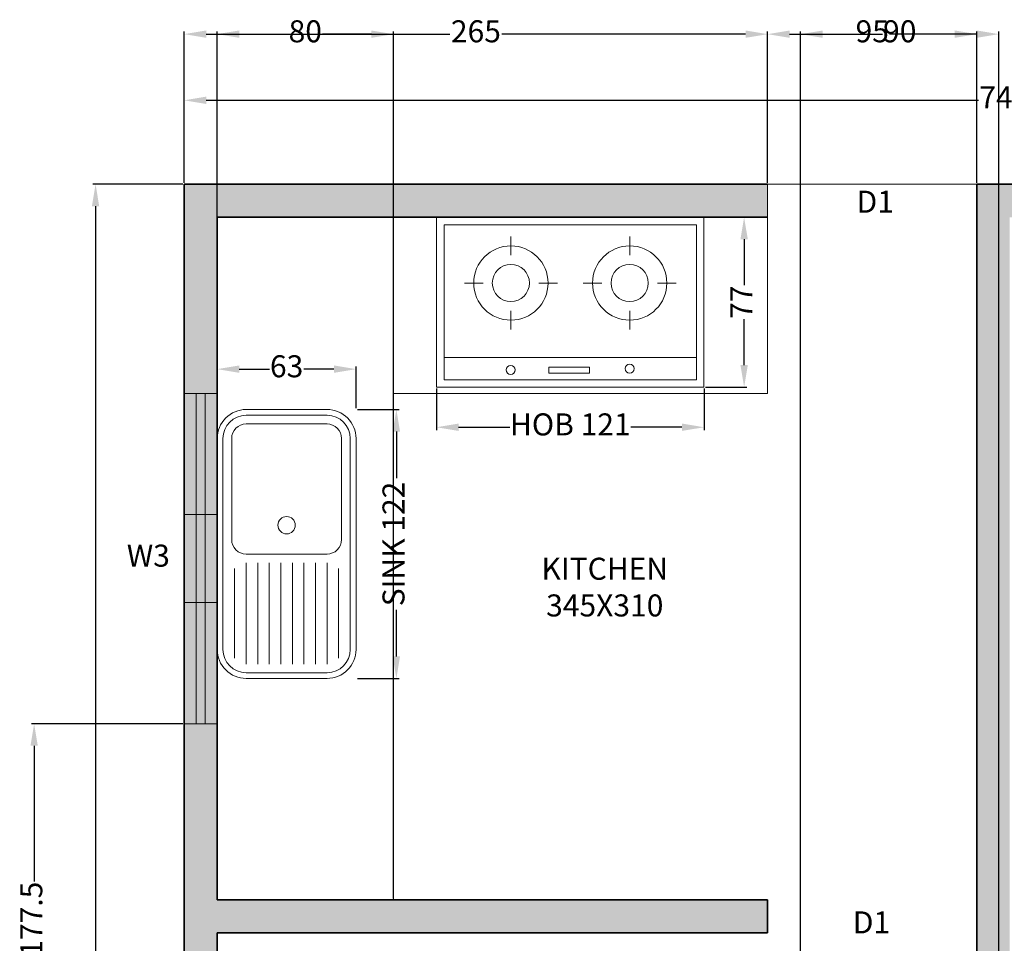
# Model space of a CAD drawing. Units: centimetres. Extents: x 2401 to 3632, y 2122 to 3526.
# Tile 8 of 10: x 2426 to 2873, y 3106 to 3526. Entities that reach past the tile are written whole.
import ezdxf

# ---------------------------------------------------------------- set-up
doc = ezdxf.new("R2010")
doc.units = ezdxf.units.CM
for name, color, linetype, lineweight in [('A-ANNO-DIMS', 9, 'Continuous', 18), ('A-ANNO-TEXT', 9, 'Continuous', 18), ('A-AREA-IDEN', 9, 'Continuous', 25), ('A-DOOR', 4, 'Continuous', 18), ('A-FLOR-CASE', 7, 'Continuous', 18), ('A-FLOR-FIXT', 9, 'Continuous', 18), ('A-GLAZ', 4, 'Continuous', 18), ('A-WALL', 7, 'Continuous', 35), ('equipments', 9, 'Continuous', 18)]:
    doc.layers.add(name, color=color, linetype=linetype, lineweight=lineweight)
doc.layers.add('A-GLAZ-PATT', color=251, linetype='Continuous', lineweight=13, true_color=0x636466)
doc.layers.add('A-WALL-PATT', color=18, linetype='Continuous', lineweight=13, true_color=0x000000)
doc.styles.get("Standard").update_dxf_attribs({"font": 'arial.ttf'})
doc.dimstyles.new('ISO-25', dxfattribs={"dimtxt": 10, "dimasz": 10, "dimexe": 1.25, "dimexo": 0.625, "dimtad": 0, "dimtxsty": 'Standard', "dimcen": 2.5, "dimadec": 0, "dimazin": 0, "dimtfac": 1, "dimtmove": 0, "dimatfit": 3, "dimfxl": 1, "dimarcsym": 0})

# ---------------------------------------------------------------- blocks, each defined once
blk = doc.blocks.new('cooktop_2')
at = {"color": 0}
for p, q in [((2566.17, 3601.98), (2636.16, 3601.98)), ((2566.17, 3601.98), (2566.17, 3557.53)), ((2568.12, 3600.04), (2634.22, 3600.04)), ((2568.12, 3600.04), (2568.12, 3559.48)), ((2634.22, 3600.04), (2634.22, 3559.48)), ((2636.16, 3601.98), (2636.16, 3557.53)), ((2585.62, 3596.92), (2585.62, 3592.06)), ((2616.72, 3596.92), (2616.72, 3592.06)), ((2573.47, 3584.77), (2578.33, 3584.77)), ((2592.91, 3584.77), (2597.78, 3584.77)), ((2604.56, 3584.77), (2609.42, 3584.77)), ((2624.01, 3584.77), (2628.87, 3584.77)), ((2585.62, 3577.47), (2585.62, 3572.61)), ((2616.72, 3577.47), (2616.72, 3572.61)), ((2568.12, 3565.31), (2634.22, 3565.31)), ((2595.51, 3561.18), (2595.51, 3562.73)), ((2595.51, 3562.73), (2606.23, 3562.73)), ((2606.23, 3562.73), (2606.23, 3561.18)), ((2568.12, 3559.48), (2634.22, 3559.48)), ((2606.23, 3561.18), (2595.51, 3561.18)), ((2566.17, 3557.53), (2636.16, 3557.53))]:
    blk.add_line(p, q, dxfattribs=at)
for centre, radius in [((2585.62, 3584.77), 9.72), ((2616.72, 3584.77), 9.72), ((2585.62, 3584.77), 4.86), ((2616.72, 3584.77), 4.86), ((2585.57, 3562.04), 1.17), ((2616.7, 3562.38), 1.17)]:
    blk.add_circle(centre, radius, dxfattribs=at)
blk = doc.blocks.new('v')
blk.add_blockref('cooktop_2', (0, 0))
blk = doc.blocks.new('SINK_KITCHEN_SNGL')
for p, q in [((-36.5, -2), (36.5, -2)), ((-39.5, -6), (-8.5, -6)), ((-44.5, -38), (-44.5, -10)), ((-41.5, -10), (-6.5, -10)), ((44.5, -10), (44.5, -38)), ((-41.5, -14), (-6.5, -14)), ((-41.5, -18), (-6.5, -18)), ((-41.5, -22), (-6.5, -22)), ((-41.5, -26), (-6.5, -26)), ((-41.5, -30), (-6.5, -30)), ((-41.5, -34), (-6.5, -34)), ((-41.5, -38), (-6.5, -38)), ((-39.5, -42), (-8.5, -42)), ((36.5, -46), (-36.5, -46))]:
    blk.add_line(p, q)
at = {"flags": 128}
for points in [[(36.5, 0, -0.414214), (46.5, -10), (46.5, -38, -0.414214), (36.5, -48), (-36.5, -48, -0.414214), (-46.5, -38), (-46.5, -10, -0.414214), (-36.5, 0)], [(36.5, -5, -0.414214), (41.5, -10), (41.5, -38, -0.414214), (36.5, -43), (1.5, -43, -0.414214), (-3.5, -38), (-3.5, -10, -0.414214), (1.5, -5)]]:
    blk.add_lwpolyline(points, format="xyb", close=True, dxfattribs=at)
blk.add_circle((6.5, -24), 3)
for centre, start, end in [((-36.5, -10), 90, 180), ((36.5, -10), 0, 90), ((-36.5, -38), 180, 270), ((36.5, -38), 270, 0)]:
    blk.add_arc(centre, 8, start, end)
blk = doc.blocks.new('*D12')
at = {"layer": 'A-ANNO-DIMS', "color": 0, "lineweight": -2, "transparency": 16777216}
for p, q in [((2499.81, 3451.1), (2458.94, 3451.1)), ((2460.19, 3441.1), (2460.19, 2873.73)), ((2460.19, 2276.1), (2460.19, 2843.48)), ((2499.81, 2266.1), (2458.94, 2266.1))]:
    blk.add_line(p, q, dxfattribs=at)
at = {"layer": 'A-ANNO-DIMS', "color": 0, "transparency": 16777216}
for points in [[(2458.52, 3441.1), (2461.85, 3441.1), (2460.19, 3451.1)], [(2458.52, 2276.1), (2461.85, 2276.1), (2460.19, 2266.1)]]:
    blk.add_solid(points, dxfattribs=at)
at = {"layer": 'Defpoints', "color": 0, "transparency": 16777216}
for p in [(2500.44, 3451.1), (2460.19, 2266.1), (2500.44, 2266.1)]:
    blk.add_point(p, dxfattribs=at)
at = {"layer": 'A-ANNO-DIMS', "color": 0, "transparency": 16777216, "insert": (2460.19, 2858.6), "char_height": 10, "attachment_point": 5, "rotation": 90}
blk.add_mtext('1185', dxfattribs=at)
blk = doc.blocks.new('*D17')
at = {"layer": 'A-ANNO-DIMS', "color": 0, "lineweight": -2, "transparency": 16777216}
for p, q in [((2500.44, 3451.73), (2500.44, 3490.46)), ((2510.44, 3489.21), (2861.27, 3489.21)), ((3235.44, 3489.21), (2884.6, 3489.21)), ((3245.44, 3451.73), (3245.44, 3490.46))]:
    blk.add_line(p, q, dxfattribs=at)
at = {"layer": 'A-ANNO-DIMS', "color": 0, "transparency": 16777216}
for points in [[(2510.44, 3490.88), (2510.44, 3487.55), (2500.44, 3489.21)], [(3235.44, 3490.88), (3235.44, 3487.55), (3245.44, 3489.21)]]:
    blk.add_solid(points, dxfattribs=at)
at = {"layer": 'Defpoints', "color": 0, "transparency": 16777216}
for p in [(3245.44, 3489.21), (2500.44, 3451.1), (3245.44, 3451.1)]:
    blk.add_point(p, dxfattribs=at)
at = {"layer": 'A-ANNO-DIMS', "color": 0, "transparency": 16777216, "insert": (2872.94, 3489.21), "char_height": 10, "attachment_point": 5}
blk.add_mtext('745', dxfattribs=at)
blk = doc.blocks.new('WIN-1500-3P')
for p, q in [((0, 15), (0, 0)), ((55, 15), (55, 0)), ((95, 15), (95, 0)), ((150, 15), (150, 0)), ((0, 9.5), (150, 9.5)), ((0, 5.5), (150, 5.5))]:
    blk.add_line(p, q)
blk = doc.blocks.new('*D28')
at = {"layer": 'A-ANNO-DIMS', "color": 0, "lineweight": -2, "transparency": 16777216}
for p, q in [((2615.07, 3358.34), (2615.07, 3339.49)), ((2736.54, 3358.34), (2736.54, 3339.49)), ((2625.07, 3340.74), (2648.29, 3340.74)), ((2726.54, 3340.74), (2703.32, 3340.74))]:
    blk.add_line(p, q, dxfattribs=at)
at = {"layer": 'A-ANNO-DIMS', "color": 0, "transparency": 16777216}
for points in [[(2625.07, 3342.41), (2625.07, 3339.08), (2615.07, 3340.74)], [(2726.54, 3342.41), (2726.54, 3339.08), (2736.54, 3340.74)]]:
    blk.add_solid(points, dxfattribs=at)
at = {"layer": 'Defpoints', "color": 0, "transparency": 16777216}
for p in [(2615.07, 3358.97), (2736.54, 3358.97), (2736.54, 3340.74)]:
    blk.add_point(p, dxfattribs=at)
at = {"layer": 'A-ANNO-DIMS', "color": 0, "transparency": 16777216, "insert": (2675.81, 3340.74), "char_height": 10, "attachment_point": 5}
blk.add_mtext('HOB 121', dxfattribs=at)
blk = doc.blocks.new('*D29')
at = {"layer": 'A-ANNO-DIMS', "color": 0, "lineweight": -2, "transparency": 16777216}
for p, q in [((2737.16, 3436.1), (2756.01, 3436.1)), ((2754.76, 3426.1), (2754.76, 3405.28)), ((2754.76, 3368.97), (2754.76, 3389.79)), ((2737.16, 3358.97), (2756.01, 3358.97))]:
    blk.add_line(p, q, dxfattribs=at)
at = {"layer": 'A-ANNO-DIMS', "color": 0, "transparency": 16777216}
for points in [[(2753.09, 3426.1), (2756.43, 3426.1), (2754.76, 3436.1)], [(2753.09, 3368.97), (2756.43, 3368.97), (2754.76, 3358.97)]]:
    blk.add_solid(points, dxfattribs=at)
at = {"layer": 'Defpoints', "color": 0, "transparency": 16777216}
for p in [(2736.54, 3436.1), (2754.76, 3436.1), (2736.54, 3358.97)]:
    blk.add_point(p, dxfattribs=at)
at = {"layer": 'A-ANNO-DIMS', "color": 0, "transparency": 16777216, "insert": (2754.76, 3397.53), "char_height": 10, "attachment_point": 5, "rotation": 90}
blk.add_mtext('77', dxfattribs=at)
blk = doc.blocks.new('*D30')
at = {"layer": 'A-ANNO-DIMS', "color": 0, "lineweight": -2, "transparency": 16777216}
for p, q in [((2579.1, 3348.81), (2598.05, 3348.81)), ((2596.8, 3338.81), (2596.8, 3317.58)), ((2596.8, 3236.66), (2596.8, 3257.89)), ((2579.1, 3226.66), (2598.05, 3226.66))]:
    blk.add_line(p, q, dxfattribs=at)
at = {"layer": 'A-ANNO-DIMS', "color": 0, "transparency": 16777216}
for points in [[(2595.14, 3338.81), (2598.47, 3338.81), (2596.8, 3348.81)], [(2595.14, 3236.66), (2598.47, 3236.66), (2596.8, 3226.66)]]:
    blk.add_solid(points, dxfattribs=at)
at = {"layer": 'Defpoints', "color": 0, "transparency": 16777216}
for p in [(2578.48, 3348.81), (2596.8, 3348.81), (2578.48, 3226.66)]:
    blk.add_point(p, dxfattribs=at)
at = {"layer": 'A-ANNO-DIMS', "color": 0, "transparency": 16777216, "insert": (2596.8, 3287.73), "char_height": 10, "attachment_point": 5, "rotation": 90}
blk.add_mtext('SINK 122', dxfattribs=at)
blk = doc.blocks.new('*D31')
at = {"layer": 'A-ANNO-DIMS', "color": 0, "lineweight": -2, "transparency": 16777216}
for p, q in [((2515.44, 3349.43), (2515.44, 3368.38)), ((2578.48, 3349.43), (2578.48, 3368.38)), ((2525.44, 3367.13), (2539.14, 3367.13)), ((2568.48, 3367.13), (2554.77, 3367.13))]:
    blk.add_line(p, q, dxfattribs=at)
at = {"layer": 'A-ANNO-DIMS', "color": 0, "transparency": 16777216}
for points in [[(2525.44, 3368.8), (2525.44, 3365.46), (2515.44, 3367.13)], [(2568.48, 3368.8), (2568.48, 3365.46), (2578.48, 3367.13)]]:
    blk.add_solid(points, dxfattribs=at)
at = {"layer": 'Defpoints', "color": 0, "transparency": 16777216}
for p in [(2515.44, 3367.13), (2515.44, 3348.81), (2578.48, 3348.81)]:
    blk.add_point(p, dxfattribs=at)
at = {"layer": 'A-ANNO-DIMS', "color": 0, "transparency": 16777216, "insert": (2546.96, 3367.13), "char_height": 10, "attachment_point": 5}
blk.add_mtext('63', dxfattribs=at)
blk = doc.blocks.new('*D42')
at = {"layer": 'A-ANNO-DIMS', "color": 0, "lineweight": -2, "transparency": 16777216}
for p, q in [((2499.81, 3206.1), (2431.04, 3206.1)), ((2432.29, 3196.1), (2432.29, 3134.42)), ((2432.29, 3038.6), (2432.29, 3100.29)), ((2499.81, 3028.6), (2431.04, 3028.6))]:
    blk.add_line(p, q, dxfattribs=at)
at = {"layer": 'A-ANNO-DIMS', "color": 0, "transparency": 16777216}
for points in [[(2430.62, 3196.1), (2433.95, 3196.1), (2432.29, 3206.1)], [(2430.62, 3038.6), (2433.95, 3038.6), (2432.29, 3028.6)]]:
    blk.add_solid(points, dxfattribs=at)
at = {"layer": 'Defpoints', "color": 0, "transparency": 16777216}
for p in [(2432.29, 3206.1), (2500.44, 3206.1), (2500.44, 3028.6)]:
    blk.add_point(p, dxfattribs=at)
at = {"layer": 'A-ANNO-DIMS', "color": 0, "transparency": 16777216, "insert": (2432.29, 3117.35), "char_height": 10, "attachment_point": 5, "rotation": 90}
blk.add_mtext('177.5', dxfattribs=at)
blk = doc.blocks.new('*D48')
at = {"layer": 'A-ANNO-DIMS', "color": 0, "lineweight": -2, "transparency": 16777216}
for p, q in [((2765.44, 3451.73), (2765.44, 3520.5)), ((2860.44, 3451.73), (2860.44, 3520.5)), ((2775.44, 3519.25), (2805.11, 3519.25)), ((2850.44, 3519.25), (2820.76, 3519.25))]:
    blk.add_line(p, q, dxfattribs=at)
at = {"layer": 'A-ANNO-DIMS', "color": 0, "transparency": 16777216}
for points in [[(2775.44, 3520.92), (2775.44, 3517.59), (2765.44, 3519.25)], [(2850.44, 3520.92), (2850.44, 3517.59), (2860.44, 3519.25)]]:
    blk.add_solid(points, dxfattribs=at)
at = {"layer": 'Defpoints', "color": 0, "transparency": 16777216}
for p in [(2860.44, 3519.25), (2765.44, 3451.1), (2860.44, 3451.1)]:
    blk.add_point(p, dxfattribs=at)
at = {"layer": 'A-ANNO-DIMS', "color": 0, "transparency": 16777216, "insert": (2812.94, 3519.25), "char_height": 10, "attachment_point": 5}
blk.add_mtext('95', dxfattribs=at)
blk = doc.blocks.new('*D49')
at = {"layer": 'A-ANNO-DIMS', "color": 0, "lineweight": -2, "transparency": 16777216}
for p, q in [((2500.44, 3451.73), (2500.44, 3520.5)), ((2765.44, 3451.73), (2765.44, 3520.5)), ((2510.44, 3519.25), (2621.14, 3519.25)), ((2755.44, 3519.25), (2644.73, 3519.25))]:
    blk.add_line(p, q, dxfattribs=at)
at = {"layer": 'A-ANNO-DIMS', "color": 0, "transparency": 16777216}
for points in [[(2510.44, 3520.92), (2510.44, 3517.59), (2500.44, 3519.25)], [(2755.44, 3520.92), (2755.44, 3517.59), (2765.44, 3519.25)]]:
    blk.add_solid(points, dxfattribs=at)
at = {"layer": 'Defpoints', "color": 0, "transparency": 16777216}
for p in [(2765.44, 3519.25), (2500.44, 3451.1), (2765.44, 3451.1)]:
    blk.add_point(p, dxfattribs=at)
at = {"layer": 'A-ANNO-DIMS', "color": 0, "transparency": 16777216, "insert": (2632.94, 3519.25), "char_height": 10, "attachment_point": 5}
blk.add_mtext('265', dxfattribs=at)
blk = doc.blocks.new('*D51')
at = {"layer": 'A-ANNO-DIMS', "color": 0, "lineweight": -2, "transparency": 16777216}
for p, q in [((2780.44, 2796.73), (2780.44, 3520.5)), ((2870.44, 2796.73), (2870.44, 3520.5)), ((2790.44, 3519.25), (2817.67, 3519.25)), ((2860.44, 3519.25), (2833.21, 3519.25))]:
    blk.add_line(p, q, dxfattribs=at)
at = {"layer": 'A-ANNO-DIMS', "color": 0, "transparency": 16777216}
for points in [[(2790.44, 3520.92), (2790.44, 3517.59), (2780.44, 3519.25)], [(2860.44, 3520.92), (2860.44, 3517.59), (2870.44, 3519.25)]]:
    blk.add_solid(points, dxfattribs=at)
at = {"layer": 'Defpoints', "color": 0, "transparency": 16777216}
for p in [(2870.44, 3519.25), (2780.44, 2796.1), (2870.44, 2796.1)]:
    blk.add_point(p, dxfattribs=at)
at = {"layer": 'A-ANNO-DIMS', "color": 0, "transparency": 16777216, "insert": (2825.44, 3519.25), "char_height": 10, "attachment_point": 5}
blk.add_mtext('90', dxfattribs=at)
blk = doc.blocks.new('*D53')
at = {"layer": 'A-ANNO-DIMS', "color": 0, "lineweight": -2, "transparency": 16777216}
for p, q in [((2515.44, 3126.73), (2515.44, 3520.5)), ((2595.44, 3126.73), (2595.44, 3520.5)), ((2525.44, 3519.25), (2547.66, 3519.25)), ((2585.44, 3519.25), (2563.21, 3519.25))]:
    blk.add_line(p, q, dxfattribs=at)
at = {"layer": 'A-ANNO-DIMS', "color": 0, "transparency": 16777216}
for points in [[(2525.44, 3520.92), (2525.44, 3517.59), (2515.44, 3519.25)], [(2585.44, 3520.92), (2585.44, 3517.59), (2595.44, 3519.25)]]:
    blk.add_solid(points, dxfattribs=at)
at = {"layer": 'Defpoints', "color": 0, "transparency": 16777216}
for p in [(2595.44, 3519.25), (2515.44, 3126.1), (2595.44, 3126.1)]:
    blk.add_point(p, dxfattribs=at)
at = {"layer": 'A-ANNO-DIMS', "color": 0, "transparency": 16777216, "insert": (2555.44, 3519.25), "char_height": 10, "attachment_point": 5}
blk.add_mtext('80', dxfattribs=at)

msp = doc.modelspace()

# ---------------------------------------------------------------- hatches: boundary and pattern name
at = {"layer": 'A-GLAZ-PATT'}
h = msp.add_hatch(color=256, dxfattribs=at)
h.dxf.hatch_style = 1
h.paths.add_polyline_path([(2505.936, 3356.104), (2500.436, 3356.104), (2500.436, 3301.104), (2505.936, 3301.104)])
h.paths.add_polyline_path([(2509.936, 3356.104), (2505.936, 3356.104), (2505.936, 3301.104), (2509.936, 3301.104)])
h.paths.add_polyline_path([(2515.436, 3335.674), (2515.436, 3356.104), (2509.936, 3356.104), (2509.936, 3301.104), (2515.436, 3301.104)])
h.paths.add_polyline_path([(2509.936, 3301.104), (2505.936, 3301.104), (2505.936, 3261.104), (2509.936, 3261.104)])
h.paths.add_polyline_path([(2515.436, 3301.104), (2509.936, 3301.104), (2509.936, 3261.104), (2515.436, 3261.104)])
h.paths.add_polyline_path([(2505.936, 3301.104), (2500.436, 3301.104), (2500.436, 3261.104), (2505.936, 3261.104)])
h.paths.add_polyline_path([(2515.436, 3261.104), (2509.936, 3261.104), (2509.936, 3206.104), (2515.436, 3206.104)])
h.paths.add_polyline_path([(2505.936, 3261.104), (2500.436, 3261.104), (2500.436, 3206.104), (2505.936, 3206.104)])
h.paths.add_polyline_path([(2509.936, 3261.104), (2505.936, 3261.104), (2505.936, 3206.104), (2509.936, 3206.104)])
h.paths.add_polyline_path([(3127.936, 3451.104), (3072.936, 3451.104), (3072.936, 3445.604), (3127.936, 3445.604)])
h.paths.add_polyline_path([(3032.936, 3441.604), (2977.936, 3441.604), (2977.936, 3436.104), (3032.936, 3436.104)])
h.paths.add_polyline_path([(3032.936, 3451.104), (2977.936, 3451.104), (2977.936, 3445.604), (3032.936, 3445.604)])
h.paths.add_polyline_path([(3032.936, 3445.604), (2977.936, 3445.604), (2977.936, 3441.604), (3032.936, 3441.604)])
h.paths.add_polyline_path([(3072.936, 3451.104), (3032.936, 3451.104), (3032.936, 3445.604), (3072.936, 3445.604)])
h.paths.add_polyline_path([(3072.936, 3445.604), (3032.936, 3445.604), (3032.936, 3441.604), (3072.936, 3441.604)])
h.paths.add_polyline_path([(3072.936, 3441.604), (3032.936, 3441.604), (3032.936, 3436.104), (3072.936, 3436.104)])
h.paths.add_polyline_path([(3127.936, 3441.604), (3072.936, 3441.604), (3072.936, 3436.104), (3127.936, 3436.104)])
h.paths.add_polyline_path([(3127.936, 3445.604), (3072.936, 3445.604), (3072.936, 3441.604), (3127.936, 3441.604)])
h.paths.add_polyline_path([(3245.436, 3356.104), (3239.936, 3356.104), (3239.936, 3301.104), (3245.436, 3301.104)])
h.paths.add_polyline_path([(3239.936, 3356.104), (3235.936, 3356.104), (3235.936, 3301.104), (3239.936, 3301.104)])
h.paths.add_polyline_path([(3235.936, 3356.104), (3230.436, 3356.104), (3230.436, 3301.104), (3235.936, 3301.104)])
h.paths.add_polyline_path([(3235.936, 3301.104), (3230.436, 3301.104), (3230.436, 3261.104), (3235.936, 3261.104)])
h.paths.add_polyline_path([(3239.936, 3301.104), (3235.936, 3301.104), (3235.936, 3261.104), (3239.936, 3261.104)])
h.paths.add_polyline_path([(3245.436, 3301.104), (3239.936, 3301.104), (3239.936, 3261.104), (3245.436, 3261.104)])
h.paths.add_polyline_path([(3245.436, 3261.104), (3239.936, 3261.104), (3239.936, 3206.104), (3245.436, 3206.104)])
h.paths.add_polyline_path([(3239.936, 3261.104), (3235.936, 3261.104), (3235.936, 3206.104), (3239.936, 3206.104)])
h.paths.add_polyline_path([(3235.936, 3261.104), (3230.436, 3261.104), (3230.436, 3206.104), (3235.936, 3206.104)])
h.paths.add_polyline_path([(3239.936, 3036.104), (3235.936, 3036.104), (3235.936, 2976.104), (3239.936, 2976.104)])
h.paths.add_polyline_path([(3235.936, 3036.104), (3230.436, 3036.104), (3230.436, 2976.104), (3235.936, 2976.104)])
h.paths.add_polyline_path([(3245.436, 3036.104), (3239.936, 3036.104), (3239.936, 2976.104), (3245.436, 2976.104)])
h.paths.add_polyline_path([(3235.936, 2836.104), (3230.436, 2836.104), (3230.436, 2781.104), (3235.936, 2781.104)])
h.paths.add_polyline_path([(3245.436, 2836.104), (3239.936, 2836.104), (3239.936, 2781.104), (3245.436, 2781.104)])
h.paths.add_polyline_path([(3239.936, 2836.104), (3235.936, 2836.104), (3235.936, 2781.104), (3239.936, 2781.104)])
h.paths.add_polyline_path([(3245.436, 2781.104), (3239.936, 2781.104), (3239.936, 2741.104), (3245.436, 2741.104)])
h.paths.add_polyline_path([(3239.936, 2781.104), (3235.936, 2781.104), (3235.936, 2741.104), (3239.936, 2741.104)])
h.paths.add_polyline_path([(3235.936, 2781.104), (3230.436, 2781.104), (3230.436, 2741.104), (3235.936, 2741.104)])
h.paths.add_polyline_path([(3245.436, 2741.104), (3239.936, 2741.104), (3239.936, 2686.104), (3245.436, 2686.104)])
h.paths.add_polyline_path([(3239.936, 2741.104), (3235.936, 2741.104), (3235.936, 2686.104), (3239.936, 2686.104)])
h.paths.add_polyline_path([(3235.936, 2741.104), (3230.436, 2741.104), (3230.436, 2686.104), (3235.936, 2686.104)])
h.paths.add_polyline_path([(3187.936, 2606.104), (3132.936, 2606.104), (3132.936, 2600.604), (3187.936, 2600.604)])
h.paths.add_polyline_path([(3187.936, 2600.604), (3132.936, 2600.604), (3132.936, 2596.604), (3187.936, 2596.604)])
h.paths.add_polyline_path([(3187.936, 2596.604), (3132.936, 2596.604), (3132.936, 2591.104), (3187.936, 2591.104)])
h.paths.add_polyline_path([(3132.936, 2596.604), (3092.936, 2596.604), (3092.936, 2591.104), (3132.936, 2591.104)])
h.paths.add_polyline_path([(3132.936, 2600.604), (3092.936, 2600.604), (3092.936, 2596.604), (3132.936, 2596.604)])
h.paths.add_polyline_path([(3132.936, 2606.104), (3092.936, 2606.104), (3092.936, 2600.604), (3132.936, 2600.604)])
h.paths.add_polyline_path([(3092.936, 2596.604), (3037.936, 2596.604), (3037.936, 2591.104), (3092.936, 2591.104)])
h.paths.add_polyline_path([(3092.936, 2600.604), (3037.936, 2600.604), (3037.936, 2596.604), (3092.936, 2596.604)])
h.paths.add_polyline_path([(3092.936, 2606.104), (3037.936, 2606.104), (3037.936, 2600.604), (3092.936, 2600.604)])
h.paths.add_polyline_path([(2803.613, 3432.66), (2826.471, 3432.66), (2826.471, 3453.267), (2803.613, 3453.267)], flags=9)
h.paths.add_polyline_path([(2904.038, 3087.418), (2926.896, 3087.418), (2926.896, 3108.025), (2904.038, 3108.025)], flags=9)
h.paths.add_polyline_path([(2801.908, 3105.391), (2824.766, 3105.391), (2824.766, 3125.998), (2801.908, 3125.998)], flags=9)
h.paths.add_polyline_path([(2757.576, 2660.284), (2780.434, 2660.284), (2780.434, 2680.892), (2757.576, 2680.892)], flags=9)
h.paths.add_polyline_path([(3004.446, 3080.825), (3027.304, 3080.825), (3027.304, 3101.432), (3004.446, 3101.432)], flags=9)
h.paths.add_polyline_path([(2805.63, 2777.019), (2828.489, 2777.019), (2828.489, 2797.626), (2805.63, 2797.626)], flags=9)
h.paths.add_polyline_path([(3094.334, 2572.754), (3128.823, 2572.754), (3128.823, 2593.361), (3094.334, 2593.361)], flags=9)
h.paths.add_polyline_path([(2931.792, 2588.154), (2946.88, 2588.154), (2946.88, 2608.761), (2931.792, 2608.761)], flags=9)
h.paths.add_polyline_path([(2582.951, 2415.87), (2664.015, 2415.87), (2664.015, 2453.184), (2582.951, 2453.184)], flags=9)
h.paths.add_polyline_path([(2622.234, 2685.113), (2683.168, 2685.113), (2683.168, 2722.427), (2622.234, 2722.427)], flags=9)
h.paths.add_polyline_path([(3027.646, 2511.408), (3088.58, 2511.408), (3088.58, 2548.722), (3027.646, 2548.722)], flags=9)
h.paths.add_polyline_path([(3020.004, 2720.966), (3092.521, 2720.966), (3092.521, 2758.281), (3020.004, 2758.281)], flags=9)
h.paths.add_polyline_path([(2628.506, 2930.416), (2689.441, 2930.416), (2689.441, 2967.73), (2628.506, 2967.73)], flags=9)
h.paths.add_polyline_path([(3056.573, 2986.666), (3117.507, 2986.666), (3117.507, 3023.981), (3056.573, 3023.981)], flags=9)
h.paths.add_polyline_path([(3083.425, 3281.357), (3164.489, 3281.357), (3164.489, 3318.672), (3083.425, 3318.672)], flags=9)
h.paths.add_polyline_path([(2658.367, 3249.15), (2724.683, 3249.15), (2724.683, 3286.465), (2658.367, 3286.465)], flags=9)
at = {"layer": 'A-WALL-PATT'}
h = msp.add_hatch(color=256, dxfattribs=at)
h.dxf.hatch_style = 1
h.paths.add_polyline_path([(2765.436, 3451.104), (2500.436, 3451.104), (2500.436, 3356.104), (2515.436, 3356.104), (2515.436, 3436.104), (2765.436, 3436.104)])
h.paths.add_polyline_path([(3245.436, 3451.104), (3127.936, 3451.104), (3127.936, 3436.104), (3185.226, 3436.104), (3185.226, 3436.735), (3230.436, 3436.735), (3230.436, 3356.104), (3245.436, 3356.104)])
h.paths.add_polyline_path([(3245.436, 2686.104), (3230.436, 2686.104), (3230.436, 2606.104), (3187.936, 2606.104), (3187.936, 2591.104), (3245.436, 2591.104)])
h.paths.add_polyline_path([(3037.936, 2606.104), (2995.436, 2606.104), (2995.436, 2591.104), (3037.936, 2591.104)])
h.paths.add_polyline_path([(3245.436, 2976.104), (3230.436, 2976.104), (3230.436, 2931.104), (2980.436, 2931.104), (2980.436, 3096.104), (2965.436, 3096.104), (2965.436, 2916.104), (3230.436, 2916.104), (3230.436, 2836.104), (3245.436, 2836.104)])
h.paths.add_polyline_path([(3230.436, 3096.104), (3055.436, 3096.104), (3055.436, 3081.104), (3230.436, 3081.104)], flags=17)
h.paths.add_polyline_path([(2977.936, 3451.104), (2860.436, 3451.104), (2860.436, 3096.104), (2875.436, 3096.104), (2875.436, 3436.104), (2977.936, 3436.104)])
h.paths.add_polyline_path([(2765.436, 3126.104), (2515.436, 3126.104), (2515.436, 3206.104), (2500.436, 3206.104), (2500.436, 3028.604), (2515.436, 3028.604), (2515.436, 3111.104), (2765.436, 3111.104)])
h.paths.add_polyline_path([(2780.436, 2796.104), (2515.436, 2796.104), (2515.436, 2878.604), (2500.436, 2878.604), (2500.436, 2736.104), (2515.436, 2736.104), (2515.436, 2781.104), (2765.436, 2781.104), (2765.436, 2706.104), (2780.436, 2706.104)])
h.paths.add_polyline_path([(2780.436, 2631.104), (2515.436, 2631.104), (2515.436, 2676.104), (2500.436, 2676.104), (2500.436, 2523.604), (2515.436, 2523.604), (2515.436, 2616.104), (2780.436, 2616.104)])
h.paths.add_polyline_path([(2885.436, 2796.104), (2870.436, 2796.104), (2870.436, 2281.104), (2762.936, 2281.104), (2762.936, 2266.104), (2885.436, 2266.104)])
h.paths.add_polyline_path([(2612.936, 2281.104), (2515.436, 2281.104), (2515.436, 2373.604), (2500.436, 2373.604), (2500.436, 2266.104), (2612.936, 2266.104)])

# ---------------------------------------------------------------- linework, layer by layer
at = {"layer": 'A-DOOR'}
msp.add_line((2765.436, 3451.104), (2860.436, 3451.104), dxfattribs=at)
at = {"layer": 'A-FLOR-CASE'}
for p, q in [((2765.436, 3451.104), (2765.436, 3356.104)), ((2765.436, 3356.104), (2595.436, 3356.104)), ((2595.436, 3356.104), (2595.436, 3126.104))]:
    msp.add_line(p, q, dxfattribs=at)
at = {"layer": 'A-WALL'}
for p, q in [((2860.436, 3451.104), (2860.436, 3096.104)), ((2515.436, 3436.104), (2515.436, 3126.104)), ((2765.436, 3436.104), (2515.436, 3436.104)), ((2765.436, 3126.104), (2515.436, 3126.104)), ((2765.436, 3126.104), (2765.436, 3111.104)), ((2765.436, 3126.104), (2765.436, 3111.104)), ((2765.436, 3111.104), (2515.436, 3111.104)), ((2515.436, 3111.104), (2515.436, 2796.104))]:
    msp.add_line(p, q, dxfattribs=at)
for points in [[(2765.436, 3451.104), (2500.436, 3451.104), (2500.436, 2266.104), (2885.436, 2266.104), (2885.436, 2796.104)], [(2885.436, 2411.104), (3245.436, 2411.104), (3245.436, 3451.104), (2860.436, 3451.104)]]:
    msp.add_lwpolyline(points, dxfattribs=at)

# ---------------------------------------------------------------- block references
at = {"layer": 'A-FLOR-FIXT', "xscale": 1.313412975512189, "yscale": 1.313412975512189, "zscale": 1.313412975512189, "rotation": 90}
msp.add_blockref('SINK_KITCHEN_SNGL', (2515.436, 3287.735), dxfattribs=at)
at = {"layer": 'A-GLAZ', "rotation": 90.0000000000003}
msp.add_blockref('WIN-1500-3P', (2515.436, 3206.104), dxfattribs=at)
at = {"layer": 'equipments', "xscale": 1.735437004172483, "yscale": 1.735437004172483, "zscale": 1.735437004172483}
msp.add_blockref('v', (-1838.358, -2814.913), dxfattribs=at)

# ---------------------------------------------------------------- texts
at = {"layer": 'A-ANNO-TEXT', "char_height": 10, "attachment_point": 1}
for s, insert in [('\\pxqc;D1', (2781.155, 3448.161)), ('\\pxqc;W3', (2451.013, 3287.432)), ('\\pxqc;D1', (2779.45, 3120.893))]:
    msp.add_mtext_dynamic_manual_height_columns(s, width=66.28614, gutter_width=12.5, heights=[0], dxfattribs=dict(at, insert=insert))
at = {"layer": 'A-AREA-IDEN', "insert": (2658.321, 3281.489), "char_height": 10, "attachment_point": 1}
msp.add_mtext_dynamic_manual_height_columns('\\pxqc;KITCHEN\\P345X310', width=66.28614, gutter_width=12.5, heights=[0], dxfattribs=at)

# ---------------------------------------------------------------- dimensions: what is measured, and where the dimension line sits
at = {"layer": 'A-ANNO-DIMS'}
for base, p1, p2, override, picture, middle in [((2765.436, 3519.254), (2500.436, 3451.104), (2765.436, 3451.104), {"dimdec": 0, "dimlfac": 1, "dimrnd": 0, "dimzin": 0, "dimdsep": 46, "dimlunit": 2}, '*D49', (2632.936, 3519.254)), ((2595.436, 3519.254), (2515.436, 3126.104), (2595.436, 3126.104), {"dimdec": 0, "dimlfac": 1, "dimrnd": 0, "dimzin": 0, "dimdsep": 46, "dimlunit": 2}, '*D53', (2555.436, 3519.254)), ((2860.436, 3519.254), (2765.436, 3451.104), (2860.436, 3451.104), {"dimdec": 0, "dimlfac": 1, "dimrnd": 0, "dimzin": 0, "dimdsep": 46, "dimlunit": 2}, '*D48', (2812.936, 3519.254)), ((2870.436, 3519.254), (2780.436, 2796.104), (2870.436, 2796.104), {"dimdec": 0, "dimlfac": 1, "dimrnd": 0, "dimzin": 0, "dimdsep": 46, "dimlunit": 2}, '*D51', (2825.436, 3519.254)), ((3245.436, 3489.213), (2500.436, 3451.104), (3245.436, 3451.104), {"dimclrd": 0, "dimclre": 0, "dimclrt": 0}, '*D17', (2872.936, 3489.213))]:
    dim = msp.add_linear_dim(base=base, p1=p1, p2=p2, dimstyle='ISO-25', override=override, dxfattribs=at)
    dim.commit()
    dim.dimension.update_dxf_attribs({"geometry": picture, "text_midpoint": middle})
for base, p1, p2, angle, override, picture, middle in [((2460.187, 2266.104), (2500.436, 3451.104), (2500.436, 2266.104), 90, {"dimclrd": 0, "dimclre": 0, "dimclrt": 0}, '*D12', (2460.187, 2858.604)), ((2754.76, 3436.104), (2736.54, 3358.965), (2736.54, 3436.104), 90, {"dimdec": 0, "dimlfac": 1, "dimrnd": 0, "dimzin": 0, "dimdsep": 46, "dimlunit": 2}, '*D29', (2754.76, 3397.535)), ((2515.436, 3367.13), (2578.48, 3348.808), (2515.436, 3348.808), 180, {"dimdec": 0, "dimlfac": 1, "dimrnd": 0, "dimzin": 0, "dimdsep": 46, "dimlunit": 2}, '*D31', (2546.958, 3367.13)), ((2432.286, 3206.104), (2500.436, 3028.604), (2500.436, 3206.104), 90, {"dimdec": 1, "dimlfac": 1, "dimrnd": 0, "dimzin": 0, "dimdsep": 46, "dimlunit": 2}, '*D42', (2432.286, 3117.354))]:
    dim = msp.add_linear_dim(base=base, p1=p1, p2=p2, angle=angle, dimstyle='ISO-25', override=override, dxfattribs=at)
    dim.commit()
    dim.dimension.update_dxf_attribs({"geometry": picture, "text_midpoint": middle})
dim = msp.add_linear_dim(base=(2736.54, 3340.745), p1=(2615.072, 3358.965), p2=(2736.54, 3358.965), text='HOB <>', dimstyle='ISO-25', override={"dimdec": 0, "dimlfac": 1, "dimrnd": 0, "dimzin": 0, "dimdsep": 46, "dimlunit": 2}, dxfattribs=at)
dim.commit()
dim.dimension.update_dxf_attribs({"geometry": '*D28', "text_midpoint": (2675.806, 3340.745)})
dim = msp.add_linear_dim(base=(2596.802, 3348.808), p1=(2578.48, 3226.661), p2=(2578.48, 3348.808), angle=90, text='SINK <>', dimstyle='ISO-25', override={"dimdec": 0, "dimlfac": 1, "dimrnd": 0, "dimzin": 0, "dimdsep": 46, "dimlunit": 2}, dxfattribs=at)
dim.commit()
dim.dimension.update_dxf_attribs({"geometry": '*D30', "text_midpoint": (2596.802, 3287.735)})

doc.saveas('drawing.dxf')
